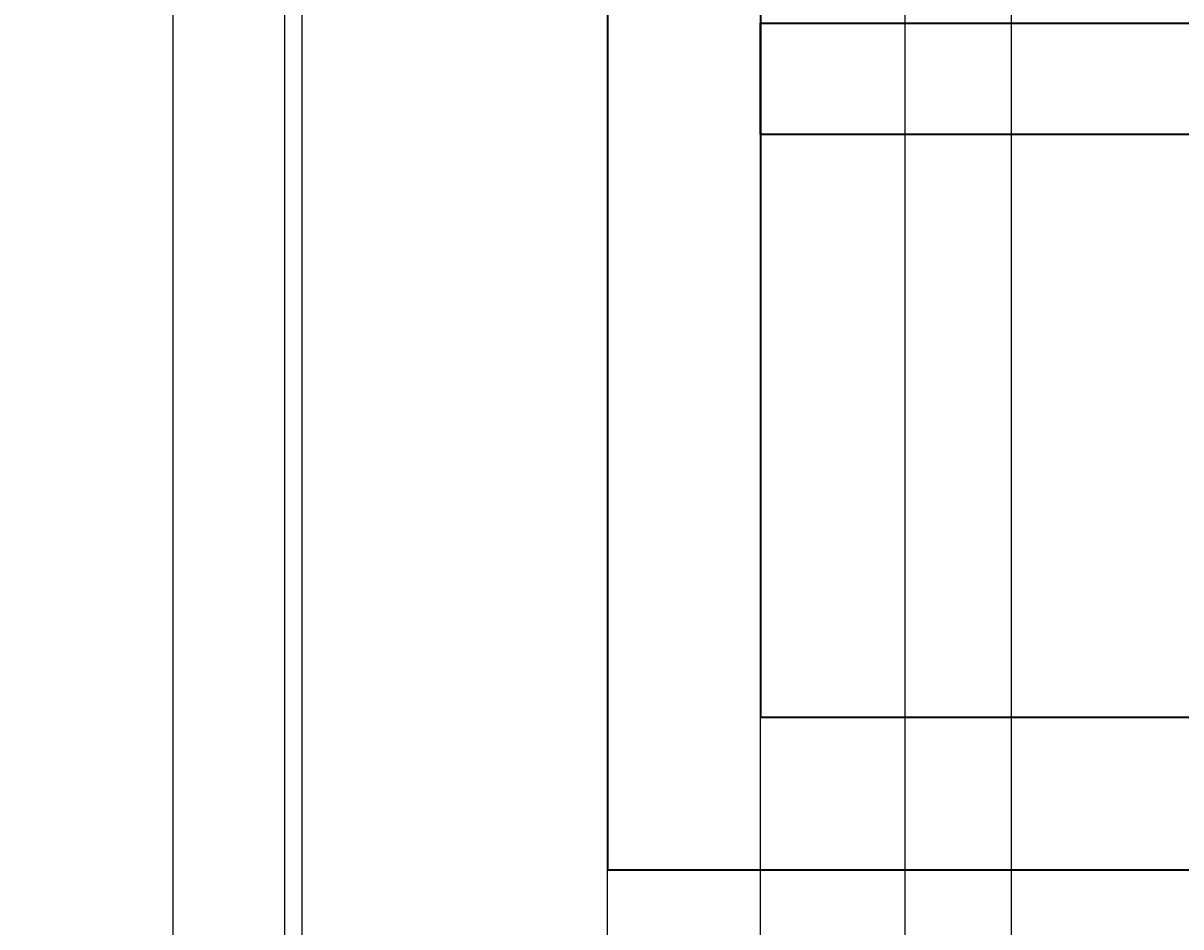
# Model space of a CAD drawing. Units: inches. Extents: x -6 to 289, y -8 to 323.
# Tile 85 of 107: x 104 to 126, y 276 to 294. Entities that reach past the tile are written whole.
import ezdxf

# ---------------------------------------------------------------- set-up
doc = ezdxf.new("R2010")
doc.units = ezdxf.units.IN
doc.header["$MEASUREMENT"] = 0
doc.layers.add('A-ANNO-DIMS', color=2, linetype='Continuous', lineweight=18)
doc.layers.add('A-ELEV', color=7, linetype='Continuous', lineweight=35)
doc.styles.get("Standard").update_dxf_attribs({"font": 'arial.ttf'})
doc.dimstyles.get("Standard").update_dxf_attribs({"dimtxt": 0.18, "dimasz": 0.18, "dimexe": 0.18, "dimexo": 0.0625, "dimgap": 0.09, "dimtad": 0, "dimtih": 1, "dimtoh": 1, "dimdec": 4, "dimzin": 0, "dimdsep": 46, "dimtxsty": 'Standard', "dimcen": 0.09, "dimadec": 0, "dimazin": 0, "dimtfac": 1, "dimtdec": 4, "dimtofl": 0, "dimtmove": 0, "dimatfit": 3, "dimfxl": 1, "dimtolj": 1, "dimtzin": 0, "dimarcsym": 0})

# ---------------------------------------------------------------- blocks, each defined once
blk = doc.blocks.new('*D9')
at = {"layer": 'A-ANNO-DIMS', "color": 0, "lineweight": -2, "transparency": 16777216}
for p, q in [((99.701, 289.105), (99.701, 322.969)), ((115.164, 307.351), (115.164, 322.969)), ((99.881, 322.789), (106.977, 322.789)), ((114.984, 322.789), (107.887, 322.789))]:
    blk.add_line(p, q, dxfattribs=at)
at = {"layer": 'A-ANNO-DIMS', "color": 0, "transparency": 16777216}
for points in [[(99.881, 322.819), (99.881, 322.759), (99.701, 322.789)], [(114.984, 322.819), (114.984, 322.759), (115.164, 322.789)]]:
    blk.add_solid(points, dxfattribs=at)
at = {"layer": 'Defpoints', "color": 0, "transparency": 16777216}
for p in [(115.164, 322.789), (115.164, 307.289), (99.701, 289.043)]:
    blk.add_point(p, dxfattribs=at)
at = {"layer": 'A-ANNO-DIMS', "color": 0, "transparency": 16777216, "insert": (107.432, 322.789), "char_height": 0.18, "attachment_point": 5}
blk.add_mtext('\\A1;15.463', dxfattribs=at)
blk = doc.blocks.new('*D10')
at = {"layer": 'A-ANNO-DIMS', "color": 0, "lineweight": -2, "transparency": 16777216}
for p, q in [((115.164, 307.351), (115.164, 322.969)), ((126.883, 226.717), (126.883, 322.969)), ((115.344, 322.789), (120.639, 322.789)), ((126.703, 322.789), (121.408, 322.789))]:
    blk.add_line(p, q, dxfattribs=at)
at = {"layer": 'A-ANNO-DIMS', "color": 0, "transparency": 16777216}
for points in [[(115.344, 322.819), (115.344, 322.759), (115.164, 322.789)], [(126.703, 322.819), (126.703, 322.759), (126.883, 322.789)]]:
    blk.add_solid(points, dxfattribs=at)
at = {"layer": 'Defpoints', "color": 0, "transparency": 16777216}
for p in [(126.883, 322.789), (115.164, 307.289), (126.883, 226.654)]:
    blk.add_point(p, dxfattribs=at)
at = {"layer": 'A-ANNO-DIMS', "color": 0, "transparency": 16777216, "insert": (121.024, 322.789), "char_height": 0.18, "attachment_point": 5}
blk.add_mtext('\\A1;11.72', dxfattribs=at)
blk = doc.blocks.new('*D27')
at = {"layer": 'A-ANNO-DIMS', "color": 0, "lineweight": -2, "transparency": 16777216}
for p, q in [((19.226, 307.289), (288.653, 307.289)), ((288.473, 307.109), (288.473, 277.471)), ((288.473, 247.469), (288.473, 277.107)), ((247.226, 247.289), (288.653, 247.289))]:
    blk.add_line(p, q, dxfattribs=at)
at = {"layer": 'A-ANNO-DIMS', "color": 0, "transparency": 16777216}
for points in [[(288.443, 307.109), (288.503, 307.109), (288.473, 307.289)], [(288.443, 247.469), (288.503, 247.469), (288.473, 247.289)]]:
    blk.add_solid(points, dxfattribs=at)
at = {"layer": 'Defpoints', "color": 0, "transparency": 16777216}
for p in [(19.164, 307.289), (288.473, 307.289), (247.164, 247.289)]:
    blk.add_point(p, dxfattribs=at)
at = {"layer": 'A-ANNO-DIMS', "color": 0, "transparency": 16777216, "insert": (288.473, 277.289), "char_height": 0.18, "attachment_point": 5}
blk.add_mtext('\\A1;60', dxfattribs=at)
blk = doc.blocks.new('*D58')
at = {"layer": 'A-ANNO-DIMS', "color": 0, "lineweight": -2, "transparency": 16777216}
for p, q in [((106.634, 68.495), (106.634, 322.969)), ((123.094, 68.495), (123.094, 322.969)), ((106.814, 322.789), (114.479, 322.789)), ((122.914, 322.789), (115.249, 322.789))]:
    blk.add_line(p, q, dxfattribs=at)
at = {"layer": 'A-ANNO-DIMS', "color": 0, "transparency": 16777216}
for points in [[(106.814, 322.819), (106.814, 322.759), (106.634, 322.789)], [(122.914, 322.819), (122.914, 322.759), (123.094, 322.789)]]:
    blk.add_solid(points, dxfattribs=at)
at = {"layer": 'Defpoints', "color": 0, "transparency": 16777216}
for p in [(123.094, 322.789), (106.634, 68.432), (123.094, 68.432)]:
    blk.add_point(p, dxfattribs=at)
at = {"layer": 'A-ANNO-DIMS', "color": 0, "transparency": 16777216, "insert": (114.864, 322.789), "char_height": 0.18, "attachment_point": 5}
blk.add_mtext('\\A1;16.46', dxfattribs=at)
blk = doc.blocks.new('*D73')
at = {"layer": 'A-ANNO-DIMS', "color": 0, "lineweight": -2, "transparency": 16777216}
for p, q in [((121.008, 51.148), (121.008, 322.969)), ((135.296, 51.148), (135.296, 322.969)), ((121.188, 322.789), (127.697, 322.789)), ((135.116, 322.789), (128.607, 322.789))]:
    blk.add_line(p, q, dxfattribs=at)
at = {"layer": 'A-ANNO-DIMS', "color": 0, "transparency": 16777216}
for points in [[(121.188, 322.819), (121.188, 322.759), (121.008, 322.789)], [(135.116, 322.819), (135.116, 322.759), (135.296, 322.789)]]:
    blk.add_solid(points, dxfattribs=at)
at = {"layer": 'Defpoints', "color": 0, "transparency": 16777216}
for p in [(135.296, 322.789), (121.008, 51.085), (135.296, 51.085)]:
    blk.add_point(p, dxfattribs=at)
at = {"layer": 'A-ANNO-DIMS', "color": 0, "transparency": 16777216, "insert": (128.152, 322.789), "char_height": 0.18, "attachment_point": 5}
blk.add_mtext('\\A1;14.288', dxfattribs=at)
blk = doc.blocks.new('*D92')
at = {"layer": 'A-ANNO-DIMS', "color": 0, "lineweight": -2, "transparency": 16777216}
for p, q in [((109.164, 127.351), (109.164, 322.969)), ((115.164, 162.411), (115.164, 322.969)), ((109.344, 322.789), (112.014, 322.789)), ((114.984, 322.789), (112.313, 322.789))]:
    blk.add_line(p, q, dxfattribs=at)
at = {"layer": 'A-ANNO-DIMS', "color": 0, "transparency": 16777216}
for points in [[(109.344, 322.819), (109.344, 322.759), (109.164, 322.789)], [(114.984, 322.819), (114.984, 322.759), (115.164, 322.789)]]:
    blk.add_solid(points, dxfattribs=at)
at = {"layer": 'Defpoints', "color": 0, "transparency": 16777216}
for p in [(115.164, 322.789), (115.164, 162.348), (109.164, 127.289)]:
    blk.add_point(p, dxfattribs=at)
at = {"layer": 'A-ANNO-DIMS', "color": 0, "transparency": 16777216, "insert": (112.164, 322.789), "char_height": 0.18, "attachment_point": 5}
blk.add_mtext('\\A1;6', dxfattribs=at)
blk = doc.blocks.new('*D93')
at = {"layer": 'A-ANNO-DIMS', "color": 0, "lineweight": -2, "transparency": 16777216}
for p, q in [((115.164, 162.411), (115.164, 322.969)), ((118.164, 159.411), (118.164, 322.969)), ((115.344, 322.789), (116.515, 322.789)), ((117.984, 322.789), (116.813, 322.789))]:
    blk.add_line(p, q, dxfattribs=at)
at = {"layer": 'A-ANNO-DIMS', "color": 0, "transparency": 16777216}
for points in [[(115.344, 322.819), (115.344, 322.759), (115.164, 322.789)], [(117.984, 322.819), (117.984, 322.759), (118.164, 322.789)]]:
    blk.add_solid(points, dxfattribs=at)
at = {"layer": 'Defpoints', "color": 0, "transparency": 16777216}
for p in [(118.164, 322.789), (115.164, 162.348), (118.164, 159.348)]:
    blk.add_point(p, dxfattribs=at)
at = {"layer": 'A-ANNO-DIMS', "color": 0, "transparency": 16777216, "insert": (116.664, 322.789), "char_height": 0.18, "attachment_point": 5}
blk.add_mtext('\\A1;3', dxfattribs=at)
blk = doc.blocks.new('*D94')
at = {"layer": 'A-ANNO-DIMS', "color": 0, "lineweight": -2, "transparency": 16777216}
for p, q in [((118.164, 159.411), (118.164, 322.969)), ((161.552, 159.411), (161.552, 322.969)), ((118.344, 322.789), (139.46, 322.789)), ((161.372, 322.789), (140.256, 322.789))]:
    blk.add_line(p, q, dxfattribs=at)
at = {"layer": 'A-ANNO-DIMS', "color": 0, "transparency": 16777216}
for points in [[(118.344, 322.819), (118.344, 322.759), (118.164, 322.789)], [(161.372, 322.819), (161.372, 322.759), (161.552, 322.789)]]:
    blk.add_solid(points, dxfattribs=at)
at = {"layer": 'Defpoints', "color": 0, "transparency": 16777216}
for p in [(161.552, 322.789), (118.164, 159.348), (161.552, 159.348)]:
    blk.add_point(p, dxfattribs=at)
at = {"layer": 'A-ANNO-DIMS', "color": 0, "transparency": 16777216, "insert": (139.858, 322.789), "char_height": 0.18, "attachment_point": 5}
blk.add_mtext('\\A1;43.39', dxfattribs=at)
blk = doc.blocks.new('*D105')
at = {"layer": 'A-ANNO-DIMS', "color": 0, "lineweight": -2, "transparency": 16777216}
for p, q in [((108.823, 259.351), (108.823, 322.969)), ((115.164, 277.105), (115.164, 322.969)), ((109.003, 322.789), (111.616, 322.789)), ((114.984, 322.789), (112.37, 322.789))]:
    blk.add_line(p, q, dxfattribs=at)
at = {"layer": 'A-ANNO-DIMS', "color": 0, "transparency": 16777216}
for points in [[(109.003, 322.819), (109.003, 322.759), (108.823, 322.789)], [(114.984, 322.819), (114.984, 322.759), (115.164, 322.789)]]:
    blk.add_solid(points, dxfattribs=at)
at = {"layer": 'Defpoints', "color": 0, "transparency": 16777216}
for p in [(115.164, 322.789), (115.164, 277.043), (108.823, 259.289)]:
    blk.add_point(p, dxfattribs=at)
at = {"layer": 'A-ANNO-DIMS', "color": 0, "transparency": 16777216, "insert": (111.993, 322.789), "char_height": 0.18, "attachment_point": 5}
blk.add_mtext('\\A1;6.341', dxfattribs=at)
blk = doc.blocks.new('*D106')
at = {"layer": 'A-ANNO-DIMS', "color": 0, "lineweight": -2, "transparency": 16777216}
for p, q in [((115.164, 277.105), (115.164, 322.969)), ((118.164, 293.728), (118.164, 322.969)), ((115.344, 322.789), (116.515, 322.789)), ((117.984, 322.789), (116.813, 322.789))]:
    blk.add_line(p, q, dxfattribs=at)
at = {"layer": 'A-ANNO-DIMS', "color": 0, "transparency": 16777216}
for points in [[(115.344, 322.819), (115.344, 322.759), (115.164, 322.789)], [(117.984, 322.819), (117.984, 322.759), (118.164, 322.789)]]:
    blk.add_solid(points, dxfattribs=at)
at = {"layer": 'Defpoints', "color": 0, "transparency": 16777216}
for p in [(118.164, 322.789), (118.164, 293.666), (115.164, 277.043)]:
    blk.add_point(p, dxfattribs=at)
at = {"layer": 'A-ANNO-DIMS', "color": 0, "transparency": 16777216, "insert": (116.664, 322.789), "char_height": 0.18, "attachment_point": 5}
blk.add_mtext('\\A1;3', dxfattribs=at)
blk = doc.blocks.new('*D107')
at = {"layer": 'A-ANNO-DIMS', "color": 0, "lineweight": -2, "transparency": 16777216}
for p, q in [((118.164, 293.728), (118.164, 322.969)), ((186.984, 291.541), (186.984, 322.969)), ((118.344, 322.789), (152.18, 322.789)), ((186.804, 322.789), (152.967, 322.789))]:
    blk.add_line(p, q, dxfattribs=at)
at = {"layer": 'A-ANNO-DIMS', "color": 0, "transparency": 16777216}
for points in [[(118.344, 322.819), (118.344, 322.759), (118.164, 322.789)], [(186.804, 322.819), (186.804, 322.759), (186.984, 322.789)]]:
    blk.add_solid(points, dxfattribs=at)
at = {"layer": 'Defpoints', "color": 0, "transparency": 16777216}
for p in [(186.984, 322.789), (118.164, 293.666), (186.984, 291.478)]:
    blk.add_point(p, dxfattribs=at)
at = {"layer": 'A-ANNO-DIMS', "color": 0, "transparency": 16777216, "insert": (152.574, 322.789), "char_height": 0.18, "attachment_point": 5}
blk.add_mtext('\\A1;68.82', dxfattribs=at)

msp = doc.modelspace()

# ---------------------------------------------------------------- linework, layer by layer
at = {"layer": 'A-ELEV'}
for points in [[(115.1638, 307.2888), (115.1638, 277.0427), (259.1638, 277.0427), (259.1638, 259.2888)], [(118.1638, 307.2888), (118.1638, 280.0427), (262.1638, 280.0427), (262.1638, 259.2888)], [(255.8036, 291.4781), (118.1638, 291.4781), (118.1638, 293.6657), (255.8036, 293.6657)]]:
    msp.add_lwpolyline(points, dxfattribs=at)

# ---------------------------------------------------------------- dimensions: what is measured, and where the dimension line sits
at = {"layer": 'A-ANNO-DIMS'}
for base, p1, p2, override, picture, middle in [((115.1638, 322.7888), (99.7007, 289.0427), (115.1638, 307.2888), {"dimdec": 3, "dimlfac": 1, "dimrnd": 0, "dimzin": 0, "dimdsep": 46, "dimlunit": 2}, '*D9', (107.4322, 322.7888)), ((123.094, 322.7888), (106.634, 68.4322), (123.094, 68.4322), {"dimdec": 2, "dimlfac": 1, "dimrnd": 0, "dimzin": 0, "dimdsep": 46, "dimlunit": 2}, '*D58', (114.864, 322.7888)), ((115.1638, 322.7888), (108.8227, 259.2888), (115.1638, 277.0427), {"dimdec": 3, "dimlfac": 1, "dimrnd": 0, "dimzin": 0, "dimdsep": 46, "dimlunit": 2}, '*D105', (111.9933, 322.7888)), ((115.1638, 322.7888), (109.1638, 127.2888), (115.1638, 162.3484), {"dimdec": 0, "dimlfac": 1, "dimrnd": 0, "dimzin": 0, "dimdsep": 46, "dimlunit": 2}, '*D92', (112.1638, 322.7888)), ((126.8835, 322.7888), (115.1638, 307.2888), (126.8835, 226.654), {"dimdec": 2, "dimlfac": 1, "dimrnd": 0, "dimzin": 0, "dimdsep": 46, "dimlunit": 2}, '*D10', (121.0236, 322.7888)), ((118.1638, 322.7888), (115.1638, 162.3484), (118.1638, 159.3484), {"dimdec": 0, "dimlfac": 1, "dimrnd": 0, "dimzin": 0, "dimdsep": 46, "dimlunit": 2}, '*D93', (116.6638, 322.7888)), ((118.1638, 322.7888), (115.1638, 277.0427), (118.1638, 293.6657), {"dimdec": 0, "dimlfac": 1, "dimrnd": 0, "dimzin": 0, "dimdsep": 46, "dimlunit": 2}, '*D106', (116.6638, 322.7888)), ((161.5522, 322.7888), (118.1638, 159.3484), (161.5522, 159.3484), {"dimdec": 2, "dimlfac": 1, "dimrnd": 0, "dimzin": 0, "dimdsep": 46, "dimlunit": 2}, '*D94', (139.858, 322.7888)), ((186.9837, 322.7888), (118.1638, 293.6657), (186.9837, 291.4781), {"dimdec": 2, "dimlfac": 1, "dimrnd": 0, "dimzin": 0, "dimdsep": 46, "dimlunit": 2}, '*D107', (152.5737, 322.7888)), ((135.296, 322.7888), (121.008, 51.0851), (135.296, 51.0851), {"dimdec": 3, "dimlfac": 1, "dimrnd": 0, "dimzin": 0, "dimdsep": 46, "dimlunit": 2}, '*D73', (128.152, 322.7888))]:
    dim = msp.add_linear_dim(base=base, p1=p1, p2=p2, dimstyle='Standard', override=override, dxfattribs=at)
    dim.commit()
    dim.dimension.update_dxf_attribs({"geometry": picture, "text_midpoint": middle})
dim = msp.add_linear_dim(base=(288.4733, 307.2888), p1=(247.1638, 247.2888), p2=(19.1638, 307.2888), angle=90, dimstyle='Standard', override={"dimdec": 0, "dimlfac": 1, "dimrnd": 0, "dimzin": 0, "dimdsep": 46, "dimlunit": 2}, dxfattribs=at)
dim.commit()
dim.dimension.update_dxf_attribs({"geometry": '*D27', "text_midpoint": (288.4733, 277.2888)})

doc.saveas('drawing.dxf')
